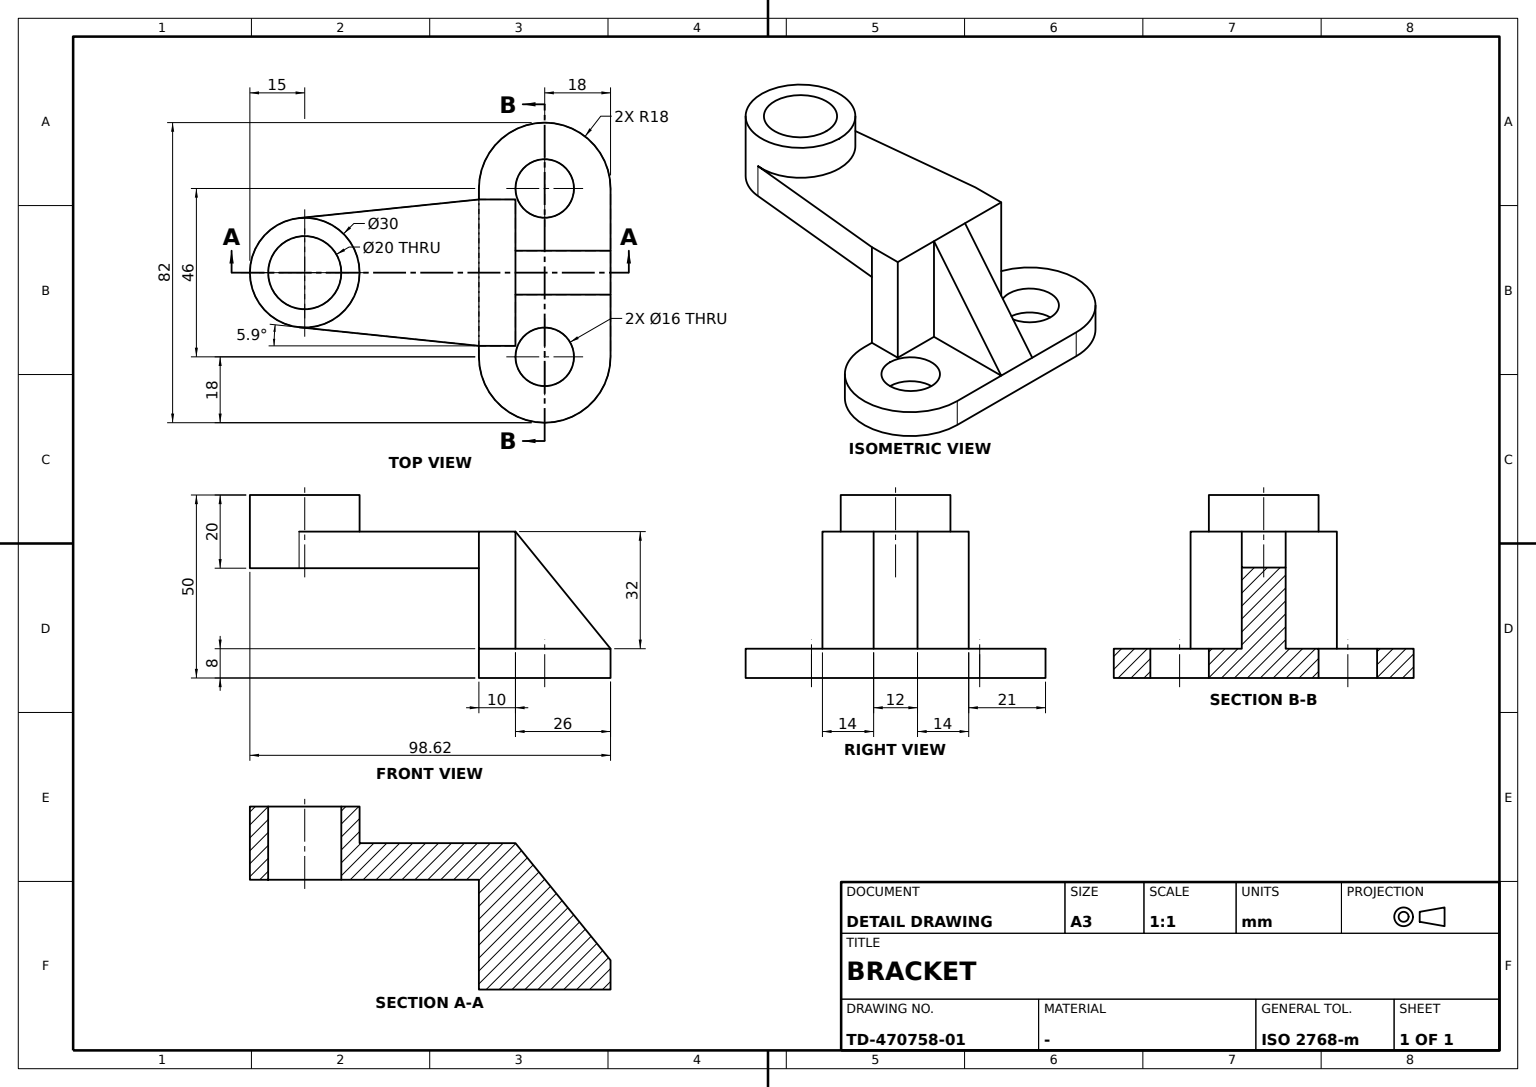
CATIA V5 part; units mm, degrees
sketch "Sketch1" plane through (0, 0, 0) normal (0, 1, 0) x (-1, 0, 0)
  line L0 (0, 0) -> (10, 0)
  line L1 (10, 0) -> (10, 32)
  line L2 (10, 32) -> (0, 32)
  line L3 (0, 32) -> (0, 0)
  dimension "length L2" = 10
  dimension "length L3" = 32
  constraint horizontal L0 x-axis
  constraint horizontal L2 x-axis
  constraint vertical L1 y-axis
  constraint vertical L3 y-axis
extrude "Pad1" add sketch "Sketch1" along normal mid plane 40
sketch "Sketch2" plane through (0, 0, 0) normal (0, 0, -1) x (1, 0, 0)
  line L0 (8, 23) -> (8, -23) construction
  point P0 (8, 23)
  point P1 (8, -23)
  line L1 (26, 23) -> (26, -23)
  line L2 (-10, -23) -> (-10, 23)
  arc A0 (26, -23) -> (-10, -23) centre (8, -23) cw
  arc A1 (-10, 23) -> (26, 23) centre (8, 23) cw
  line L3 (-10, 20) -> (-10, -20) construction
  circle A2 centre (8, 23) radius 8
  circle A3 centre (8, -23) radius 8
  dimension "distance L0 L1" = 18
  dimension "length L0" = 46
  dimension "distance L3 L2" = 0
  dimension "radius A2" = 8
  constraint vertical L0 y-axis
  constraint tangency A0 L1
  constraint tangency A1 L1
  constraint tangency A0 L2
  constraint tangency A1 L2
  constraint symmetry P0 P1 x-axis
  constraint symmetry A2 A3 x-axis
extrude "Pad2" add sketch "Sketch2" along normal blind 8
sketch "Sketch3" plane through (0, 0, 0) normal (0, 1, 0) x (-1, 0, 0)
  point P0 (0, 32)
  line L0 (0, 32) -> (0, 0)
  line L1 (0, 0) -> (-26, 0)
  point P1 (-26, 0)
  line L2 (-26, 0) -> (0, 32)
  point P2 (0, 32)
  point P3 (-26, 0)
  constraint vertical L0 y-axis
  constraint horizontal L1 x-axis
  constraint coincidence P0 P2
  constraint coincidence P1 P3
extrude "Pad3" add sketch "Sketch3" along normal mid plane 12
sketch "Sketch4" plane through (0, 0, 32) normal (0, 0, 1) x (1, 0, 0)
  circle A0 centre (-57.6207, 0) radius 10
  point P0 (-57.6207, 0)
  arc A1 (-59.1623, 14.9206) -> (-59.1623, -14.9206) centre (-57.6207, 0) ccw
  line L0 (-59.1623, 14.9206) -> (-10, 20)
  point P1 (-10, 20)
  line L1 (-59.1623, -14.9206) -> (-10, -20)
  point P2 (-10, -20)
  line L2 (-10, 20) -> (0, 20)
  point P3 (-10, 20)
  line L3 (0, 6) -> (0, 20)
  line L4 (0, -6) -> (0, 6)
  line L5 (0, -20) -> (0, -6)
  line L6 (-10, -20) -> (0, -20)
  point P4 (-10, -20)
  dimension "radius A1" = 15
  dimension "radius A0" = 10
  constraint coincidence P0 x-axis
  constraint coincidence P1 P3
  constraint coincidence P2 P4
  constraint tangency L0 A1
  constraint tangency L1 A1
extrude "Pad4" add sketch "Sketch4" against normal blind 10
sketch "Sketch5" plane through (0, 0, 32) normal (0, 0, 1) x (1, 0, 0)
  circle A0 centre (-57.6207, 0) radius 10
  circle A1 centre (-57.6207, 0) radius 15
  point P0 (-57.6207, 0)
  arc A2 (-59.1623, 14.9206) -> (-59.1623, -14.9206) centre (-57.6207, 0) ccw construction
  constraint concentricity P0 A0
  constraint coincidence A1 A2
extrude "Pad5" add sketch "Sketch5" along normal mid plane 20
properties part number "4"
